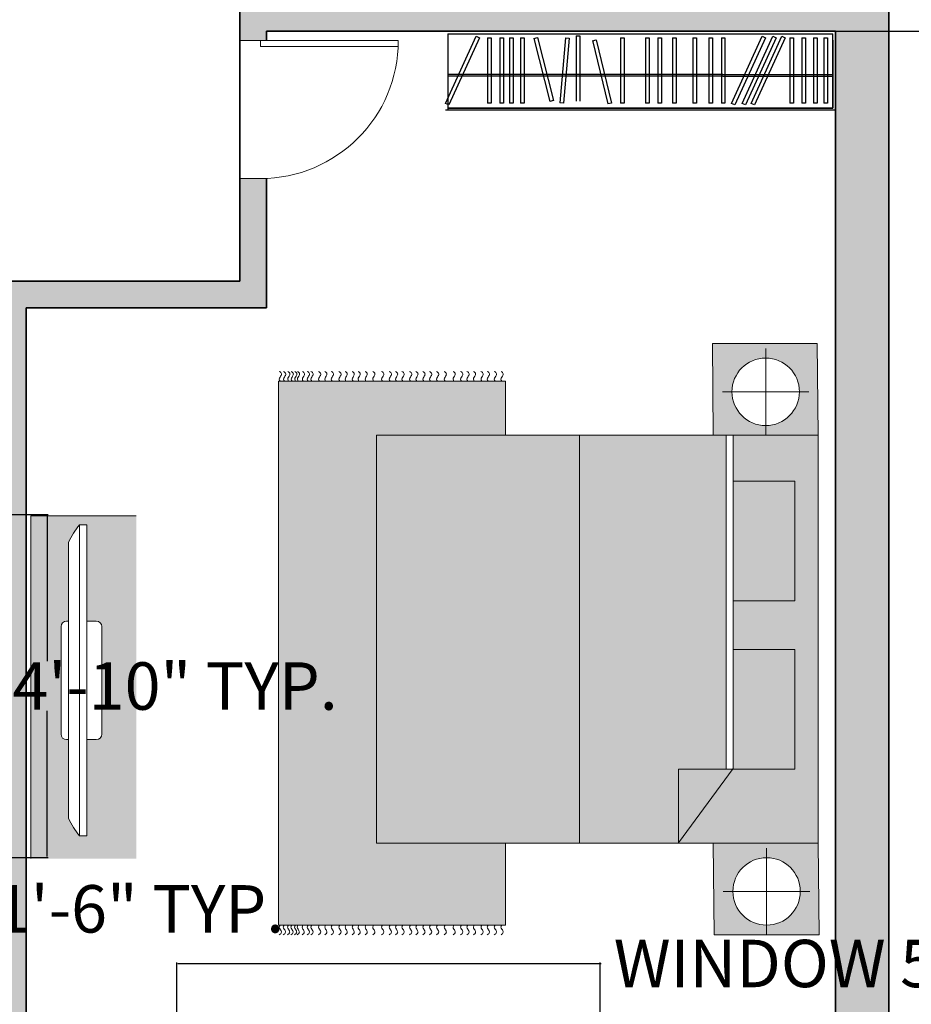
# Model space of a CAD drawing. Units: inches. Extents: x 853 to 1550, y 485 to 1596.
# Tile 7 of 18: x 1267 to 1418, y 867 to 1034. Entities that reach past the tile are written whole.
import ezdxf

# ---------------------------------------------------------------- set-up
doc = ezdxf.new("R2010")
doc.units = ezdxf.units.IN
doc.header["$MEASUREMENT"] = 0
for name, color, linetype, lineweight in [('A-ANNO-DIMS', 2, 'Continuous', 18), ('A-DOOR', 4, 'Continuous', 18), ('A-WALL-PATT', 250, 'Continuous', 13), ('closet', 32, 'Continuous', 25), ('furniture', 250, 'Continuous', 18), ('walls', 250, 'Continuous', 35)]:
    doc.layers.add(name, color=color, linetype=linetype, lineweight=lineweight)
doc.layers.add('A-FURN-PATT', color=254, linetype='Continuous', lineweight=13, true_color=0xfeeab9)
doc.styles.get("Standard").update_dxf_attribs({"font": 'arial.ttf'})
doc.dimstyles.get("Standard").update_dxf_attribs({"dimtxt": 8, "dimasz": 0.18, "dimexe": 0.18, "dimexo": 0.0625, "dimgap": 0.09, "dimtad": 0, "dimtih": 1, "dimtoh": 1, "dimzin": 0, "dimdsep": 46, "dimlunit": 3, "dimtxsty": 'Standard', "dimcen": 0.09, "dimadec": 0, "dimazin": 0, "dimtfac": 1, "dimtofl": 0, "dimtmove": 0, "dimatfit": 3, "dimfxl": 1, "dimtolj": 1, "dimtzin": 0, "dimarcsym": 0})

# ---------------------------------------------------------------- blocks, each defined once
blk = doc.blocks.new('CARPET')
at = {"layer": 'furniture'}
for p, q in [((-51.53, -98.11), (-51.53, -55.12)), ((-51.53, -55.12), (-41.27, -55.12)), ((36, -55.12), (51.55, -55.12)), ((51.55, -55.12), (51.55, -98.11)), ((51.55, -98.11), (-51.53, -98.11))]:
    blk.add_line(p, q, dxfattribs=at)
for points, knots in [([(-53.37, -55.99), (-53.22, -55.8), (-52.9, -55.41), (-52.34, -55.8), (-51.89, -56.08), (-51.65, -55.91), (-51.53, -55.83)], [0, 0, 0, 0, 0.653278, 1.290138, 1.740457, 2.114451, 2.114451, 2.114451, 2.114451]), ([(53.37, -55.99), (53.22, -55.8), (52.9, -55.41), (52.34, -55.8), (51.89, -56.08), (51.65, -55.91), (51.53, -55.83)], [0, 0, 0, 0, 0.653278, 1.290138, 1.740457, 2.114451, 2.114451, 2.114451, 2.114451]), ([(-53.37, -57.26), (-53.22, -57.07), (-52.9, -56.67), (-52.34, -57.07), (-51.89, -57.35), (-51.65, -57.17), (-51.53, -57.1)], [0, 0, 0, 0, 0.653278, 1.290138, 1.740457, 2.114451, 2.114451, 2.114451, 2.114451]), ([(53.37, -57.26), (53.22, -57.07), (52.9, -56.67), (52.34, -57.07), (51.89, -57.35), (51.65, -57.17), (51.53, -57.1)], [0, 0, 0, 0, 0.653278, 1.290138, 1.740457, 2.114451, 2.114451, 2.114451, 2.114451]), ([(-53.37, -58.59), (-53.22, -58.4), (-52.9, -58.01), (-52.34, -58.4), (-51.89, -58.68), (-51.65, -58.5), (-51.53, -58.43)], [0, 0, 0, 0, 0.653278, 1.290138, 1.740457, 2.114451, 2.114451, 2.114451, 2.114451]), ([(-53.37, -59.78), (-53.22, -59.58), (-52.9, -59.19), (-52.34, -59.58), (-51.89, -59.86), (-51.65, -59.69), (-51.53, -59.61)], [0, 0, 0, 0, 0.653278, 1.290138, 1.740457, 2.114451, 2.114451, 2.114451, 2.114451]), ([(53.37, -58.59), (53.22, -58.4), (52.9, -58.01), (52.34, -58.4), (51.89, -58.68), (51.65, -58.5), (51.53, -58.43)], [0, 0, 0, 0, 0.653278, 1.290138, 1.740457, 2.114451, 2.114451, 2.114451, 2.114451]), ([(53.37, -59.78), (53.22, -59.58), (52.9, -59.19), (52.34, -59.58), (51.89, -59.86), (51.65, -59.69), (51.53, -59.61)], [0, 0, 0, 0, 0.653278, 1.290138, 1.740457, 2.114451, 2.114451, 2.114451, 2.114451]), ([(-53.37, -61.22), (-53.22, -61.02), (-52.9, -60.63), (-52.34, -61.02), (-51.89, -61.3), (-51.65, -61.13), (-51.53, -61.05)], [0, 0, 0, 0, 0.653278, 1.290138, 1.740457, 2.114451, 2.114451, 2.114451, 2.114451]), ([(53.37, -61.22), (53.22, -61.02), (52.9, -60.63), (52.34, -61.02), (51.89, -61.3), (51.65, -61.13), (51.53, -61.05)], [0, 0, 0, 0, 0.653278, 1.290138, 1.740457, 2.114451, 2.114451, 2.114451, 2.114451]), ([(-53.37, -62.44), (-53.22, -62.25), (-52.9, -61.86), (-52.34, -62.25), (-51.89, -62.53), (-51.65, -62.36), (-51.53, -62.28)], [0, 0, 0, 0, 0.653278, 1.290138, 1.740457, 2.114451, 2.114451, 2.114451, 2.114451]), ([(-53.37, -63.63), (-53.22, -63.43), (-52.9, -63.04), (-52.34, -63.43), (-51.89, -63.72), (-51.65, -63.54), (-51.53, -63.46)], [0, 0, 0, 0, 0.653278, 1.290138, 1.740457, 2.114451, 2.114451, 2.114451, 2.114451]), ([(53.37, -62.44), (53.22, -62.25), (52.9, -61.86), (52.34, -62.25), (51.89, -62.53), (51.65, -62.36), (51.53, -62.28)], [0, 0, 0, 0, 0.653278, 1.290138, 1.740457, 2.114451, 2.114451, 2.114451, 2.114451]), ([(53.37, -63.63), (53.22, -63.43), (52.9, -63.04), (52.34, -63.43), (51.89, -63.72), (51.65, -63.54), (51.53, -63.46)], [0, 0, 0, 0, 0.653278, 1.290138, 1.740457, 2.114451, 2.114451, 2.114451, 2.114451]), ([(-53.37, -65.07), (-53.22, -64.87), (-52.9, -64.48), (-52.34, -64.87), (-51.89, -65.15), (-51.65, -64.98), (-51.53, -64.9)], [0, 0, 0, 0, 0.653278, 1.290138, 1.740457, 2.114451, 2.114451, 2.114451, 2.114451]), ([(53.37, -65.07), (53.22, -64.87), (52.9, -64.48), (52.34, -64.87), (51.89, -65.15), (51.65, -64.98), (51.53, -64.9)], [0, 0, 0, 0, 0.653278, 1.290138, 1.740457, 2.114451, 2.114451, 2.114451, 2.114451]), ([(-53.37, -66.76), (-53.22, -66.56), (-52.9, -66.17), (-52.34, -66.56), (-51.89, -66.84), (-51.65, -66.67), (-51.53, -66.59)], [0, 0, 0, 0, 0.653278, 1.290138, 1.740457, 2.114451, 2.114451, 2.114451, 2.114451]), ([(53.37, -66.76), (53.22, -66.56), (52.9, -66.17), (52.34, -66.56), (51.89, -66.84), (51.65, -66.67), (51.53, -66.59)], [0, 0, 0, 0, 0.653278, 1.290138, 1.740457, 2.114451, 2.114451, 2.114451, 2.114451]), ([(-53.37, -68.2), (-53.22, -68), (-52.9, -67.61), (-52.34, -68), (-51.89, -68.28), (-51.65, -68.11), (-51.53, -68.03)], [0, 0, 0, 0, 0.653278, 1.290138, 1.740457, 2.114451, 2.114451, 2.114451, 2.114451]), ([(53.37, -68.2), (53.22, -68), (52.9, -67.61), (52.34, -68), (51.89, -68.28), (51.65, -68.11), (51.53, -68.03)], [0, 0, 0, 0, 0.653278, 1.290138, 1.740457, 2.114451, 2.114451, 2.114451, 2.114451]), ([(-53.37, -69.53), (-53.22, -69.33), (-52.9, -68.94), (-52.34, -69.33), (-51.89, -69.61), (-51.65, -69.44), (-51.53, -69.36)], [0, 0, 0, 0, 0.653278, 1.290138, 1.740457, 2.114451, 2.114451, 2.114451, 2.114451]), ([(-53.37, -70.79), (-53.22, -70.6), (-52.9, -70.21), (-52.34, -70.6), (-51.89, -70.88), (-51.65, -70.7), (-51.53, -70.63)], [0, 0, 0, 0, 0.653278, 1.290138, 1.740457, 2.114451, 2.114451, 2.114451, 2.114451]), ([(53.37, -69.53), (53.22, -69.33), (52.9, -68.94), (52.34, -69.33), (51.89, -69.61), (51.65, -69.44), (51.53, -69.36)], [0, 0, 0, 0, 0.653278, 1.290138, 1.740457, 2.114451, 2.114451, 2.114451, 2.114451]), ([(53.37, -70.79), (53.22, -70.6), (52.9, -70.21), (52.34, -70.6), (51.89, -70.88), (51.65, -70.7), (51.53, -70.63)], [0, 0, 0, 0, 0.653278, 1.290138, 1.740457, 2.114451, 2.114451, 2.114451, 2.114451]), ([(-53.37, -72.12), (-53.22, -71.93), (-52.9, -71.54), (-52.34, -71.93), (-51.89, -72.21), (-51.65, -72.04), (-51.53, -71.96)], [0, 0, 0, 0, 0.653278, 1.290138, 1.740457, 2.114451, 2.114451, 2.114451, 2.114451]), ([(53.37, -72.12), (53.22, -71.93), (52.9, -71.54), (52.34, -71.93), (51.89, -72.21), (51.65, -72.04), (51.53, -71.96)], [0, 0, 0, 0, 0.653278, 1.290138, 1.740457, 2.114451, 2.114451, 2.114451, 2.114451]), ([(-53.37, -73.31), (-53.22, -73.11), (-52.9, -72.72), (-52.34, -73.11), (-51.89, -73.4), (-51.65, -73.22), (-51.53, -73.14)], [0, 0, 0, 0, 0.653278, 1.290138, 1.740457, 2.114451, 2.114451, 2.114451, 2.114451]), ([(-53.37, -74.75), (-53.22, -74.55), (-52.9, -74.16), (-52.34, -74.55), (-51.89, -74.83), (-51.65, -74.66), (-51.53, -74.58)], [0, 0, 0, 0, 0.653278, 1.290138, 1.740457, 2.114451, 2.114451, 2.114451, 2.114451]), ([(53.37, -73.31), (53.22, -73.11), (52.9, -72.72), (52.34, -73.11), (51.89, -73.4), (51.65, -73.22), (51.53, -73.14)], [0, 0, 0, 0, 0.653278, 1.290138, 1.740457, 2.114451, 2.114451, 2.114451, 2.114451]), ([(53.37, -74.75), (53.22, -74.55), (52.9, -74.16), (52.34, -74.55), (51.89, -74.83), (51.65, -74.66), (51.53, -74.58)], [0, 0, 0, 0, 0.653278, 1.290138, 1.740457, 2.114451, 2.114451, 2.114451, 2.114451]), ([(-53.37, -75.98), (-53.22, -75.78), (-52.9, -75.39), (-52.34, -75.78), (-51.89, -76.06), (-51.65, -75.89), (-51.53, -75.81)], [0, 0, 0, 0, 0.653278, 1.290138, 1.740457, 2.114451, 2.114451, 2.114451, 2.114451]), ([(53.37, -75.98), (53.22, -75.78), (52.9, -75.39), (52.34, -75.78), (51.89, -76.06), (51.65, -75.89), (51.53, -75.81)], [0, 0, 0, 0, 0.653278, 1.290138, 1.740457, 2.114451, 2.114451, 2.114451, 2.114451]), ([(-53.37, -77.16), (-53.22, -76.96), (-52.9, -76.57), (-52.34, -76.96), (-51.89, -77.25), (-51.65, -77.07), (-51.53, -76.99)], [0, 0, 0, 0, 0.653278, 1.290138, 1.740457, 2.114451, 2.114451, 2.114451, 2.114451]), ([(-53.37, -78.6), (-53.22, -78.4), (-52.9, -78.01), (-52.34, -78.4), (-51.89, -78.68), (-51.65, -78.51), (-51.53, -78.43)], [0, 0, 0, 0, 0.653278, 1.290138, 1.740457, 2.114451, 2.114451, 2.114451, 2.114451]), ([(53.37, -77.16), (53.22, -76.96), (52.9, -76.57), (52.34, -76.96), (51.89, -77.25), (51.65, -77.07), (51.53, -76.99)], [0, 0, 0, 0, 0.653278, 1.290138, 1.740457, 2.114451, 2.114451, 2.114451, 2.114451]), ([(53.37, -78.6), (53.22, -78.4), (52.9, -78.01), (52.34, -78.4), (51.89, -78.68), (51.65, -78.51), (51.53, -78.43)], [0, 0, 0, 0, 0.653278, 1.290138, 1.740457, 2.114451, 2.114451, 2.114451, 2.114451]), ([(-53.37, -80.29), (-53.22, -80.09), (-52.9, -79.7), (-52.34, -80.09), (-51.89, -80.37), (-51.65, -80.2), (-51.53, -80.12)], [0, 0, 0, 0, 0.653278, 1.290138, 1.740457, 2.114451, 2.114451, 2.114451, 2.114451]), ([(53.37, -80.29), (53.22, -80.09), (52.9, -79.7), (52.34, -80.09), (51.89, -80.37), (51.65, -80.2), (51.53, -80.12)], [0, 0, 0, 0, 0.653278, 1.290138, 1.740457, 2.114451, 2.114451, 2.114451, 2.114451]), ([(-53.37, -81.73), (-53.22, -81.53), (-52.9, -81.14), (-52.34, -81.53), (-51.89, -81.81), (-51.65, -81.64), (-51.53, -81.56)], [0, 0, 0, 0, 0.653278, 1.290138, 1.740457, 2.114451, 2.114451, 2.114451, 2.114451]), ([(53.37, -81.73), (53.22, -81.53), (52.9, -81.14), (52.34, -81.53), (51.89, -81.81), (51.65, -81.64), (51.53, -81.56)], [0, 0, 0, 0, 0.653278, 1.290138, 1.740457, 2.114451, 2.114451, 2.114451, 2.114451]), ([(-53.37, -83.06), (-53.22, -82.86), (-52.9, -82.47), (-52.34, -82.86), (-51.89, -83.14), (-51.65, -82.97), (-51.53, -82.89)], [0, 0, 0, 0, 0.653278, 1.290138, 1.740457, 2.114451, 2.114451, 2.114451, 2.114451]), ([(-53.37, -84.18), (-53.22, -83.99), (-52.9, -83.6), (-52.34, -83.99), (-51.89, -84.27), (-51.65, -84.09), (-51.53, -84.02)], [0, 0, 0, 0, 0.653278, 1.290138, 1.740457, 2.114451, 2.114451, 2.114451, 2.114451]), ([(53.37, -83.06), (53.22, -82.86), (52.9, -82.47), (52.34, -82.86), (51.89, -83.14), (51.65, -82.97), (51.53, -82.89)], [0, 0, 0, 0, 0.653278, 1.290138, 1.740457, 2.114451, 2.114451, 2.114451, 2.114451]), ([(53.37, -84.18), (53.22, -83.99), (52.9, -83.6), (52.34, -83.99), (51.89, -84.27), (51.65, -84.09), (51.53, -84.02)], [0, 0, 0, 0, 0.653278, 1.290138, 1.740457, 2.114451, 2.114451, 2.114451, 2.114451]), ([(-53.37, -85.51), (-53.22, -85.32), (-52.9, -84.93), (-52.34, -85.32), (-51.89, -85.6), (-51.65, -85.42), (-51.53, -85.35)], [0, 0, 0, 0, 0.653278, 1.290138, 1.740457, 2.114451, 2.114451, 2.114451, 2.114451]), ([(53.37, -85.51), (53.22, -85.32), (52.9, -84.93), (52.34, -85.32), (51.89, -85.6), (51.65, -85.42), (51.53, -85.35)], [0, 0, 0, 0, 0.653278, 1.290138, 1.740457, 2.114451, 2.114451, 2.114451, 2.114451]), ([(-53.37, -86.7), (-53.22, -86.5), (-52.9, -86.11), (-52.34, -86.5), (-51.89, -86.78), (-51.65, -86.61), (-51.53, -86.53)], [0, 0, 0, 0, 0.653278, 1.290138, 1.740457, 2.114451, 2.114451, 2.114451, 2.114451]), ([(53.37, -86.7), (53.22, -86.5), (52.9, -86.11), (52.34, -86.5), (51.89, -86.78), (51.65, -86.61), (51.53, -86.53)], [0, 0, 0, 0, 0.653278, 1.290138, 1.740457, 2.114451, 2.114451, 2.114451, 2.114451]), ([(-53.37, -88.14), (-53.22, -87.94), (-52.9, -87.55), (-52.34, -87.94), (-51.89, -88.22), (-51.65, -88.05), (-51.53, -87.97)], [0, 0, 0, 0, 0.653278, 1.290138, 1.740457, 2.114451, 2.114451, 2.114451, 2.114451]), ([(-53.37, -89.36), (-53.22, -89.17), (-52.9, -88.78), (-52.34, -89.17), (-51.89, -89.45), (-51.65, -89.28), (-51.53, -89.2)], [0, 0, 0, 0, 0.653278, 1.290138, 1.740457, 2.114451, 2.114451, 2.114451, 2.114451]), ([(53.37, -88.14), (53.22, -87.94), (52.9, -87.55), (52.34, -87.94), (51.89, -88.22), (51.65, -88.05), (51.53, -87.97)], [0, 0, 0, 0, 0.653278, 1.290138, 1.740457, 2.114451, 2.114451, 2.114451, 2.114451]), ([(53.37, -89.36), (53.22, -89.17), (52.9, -88.78), (52.34, -89.17), (51.89, -89.45), (51.65, -89.28), (51.53, -89.2)], [0, 0, 0, 0, 0.653278, 1.290138, 1.740457, 2.114451, 2.114451, 2.114451, 2.114451]), ([(-53.37, -90.55), (-53.22, -90.35), (-52.9, -89.96), (-52.34, -90.35), (-51.89, -90.64), (-51.65, -90.46), (-51.53, -90.38)], [0, 0, 0, 0, 0.653278, 1.290138, 1.740457, 2.114451, 2.114451, 2.114451, 2.114451]), ([(53.37, -90.55), (53.22, -90.35), (52.9, -89.96), (52.34, -90.35), (51.9, -90.63), (51.66, -90.47), (51.55, -90.4)], [0, 0, 0, 0, 0.653278, 1.290138, 1.740457, 2.0926, 2.0926, 2.0926, 2.0926]), ([(-53.37, -91.99), (-53.22, -91.79), (-52.9, -91.4), (-52.34, -91.79), (-51.89, -92.07), (-51.65, -91.9), (-51.53, -91.82)], [0, 0, 0, 0, 0.653278, 1.290138, 1.740457, 2.114451, 2.114451, 2.114451, 2.114451]), ([(-53.37, -92.69), (-53.22, -92.48), (-52.9, -92.08), (-52.35, -92.49), (-51.89, -92.77), (-51.65, -92.6), (-51.53, -92.52)], [0, 0, 0, 0, 0.663904, 1.307406, 1.757725, 2.131719, 2.131719, 2.131719, 2.131719]), ([(-53.37, -93.61), (-53.22, -93.42), (-52.9, -93.03), (-52.34, -93.42), (-51.89, -93.7), (-51.65, -93.52), (-51.53, -93.45)], [0, 0, 0, 0, 0.653278, 1.290138, 1.740457, 2.114451, 2.114451, 2.114451, 2.114451]), ([(53.37, -91.99), (53.22, -91.79), (52.9, -91.4), (52.34, -91.79), (51.9, -92.07), (51.66, -91.91), (51.55, -91.83)], [0, 0, 0, 0, 0.653278, 1.290138, 1.740457, 2.0926, 2.0926, 2.0926, 2.0926]), ([(53.37, -92.69), (53.22, -92.49), (52.9, -92.09), (52.34, -92.49), (51.9, -92.77), (51.66, -92.61), (51.55, -92.53)], [0, 0, 0, 0, 0.656792, 1.295826, 1.746145, 2.098292, 2.098292, 2.098292, 2.098292]), ([(53.37, -93.66), (53.22, -93.46), (52.9, -93.07), (52.34, -93.46), (51.9, -93.74), (51.66, -93.58), (51.55, -93.5)], [0, 0, 0, 0, 0.653278, 1.290138, 1.740457, 2.0926, 2.0926, 2.0926, 2.0926]), ([(-53.37, -94.55), (-53.22, -94.35), (-52.9, -93.96), (-52.34, -94.35), (-51.89, -94.63), (-51.65, -94.46), (-51.53, -94.38)], [0, 0, 0, 0, 0.653278, 1.290138, 1.740457, 2.114451, 2.114451, 2.114451, 2.114451]), ([(-53.37, -95.05), (-53.22, -94.85), (-52.9, -94.46), (-52.34, -94.85), (-51.89, -95.14), (-51.65, -94.96), (-51.53, -94.88)], [0, 0, 0, 0, 0.653278, 1.290138, 1.740457, 2.114451, 2.114451, 2.114451, 2.114451]), ([(53.37, -94.59), (53.22, -94.4), (52.9, -94.01), (52.34, -94.4), (51.9, -94.68), (51.66, -94.51), (51.55, -94.44)], [0, 0, 0, 0, 0.653278, 1.290138, 1.740457, 2.0926, 2.0926, 2.0926, 2.0926]), ([(53.37, -95.1), (53.22, -94.9), (52.9, -94.51), (52.34, -94.9), (51.9, -95.18), (51.66, -95.02), (51.55, -94.94)], [0, 0, 0, 0, 0.653278, 1.290138, 1.740457, 2.0926, 2.0926, 2.0926, 2.0926]), ([(-53.37, -95.73), (-53.22, -95.54), (-52.9, -95.15), (-52.34, -95.54), (-51.89, -95.82), (-51.65, -95.65), (-51.53, -95.57)], [0, 0, 0, 0, 0.653278, 1.290138, 1.740457, 2.114451, 2.114451, 2.114451, 2.114451]), ([(-53.37, -96.38), (-53.22, -96.18), (-52.9, -95.79), (-52.34, -96.18), (-51.89, -96.47), (-51.65, -96.29), (-51.53, -96.21)], [0, 0, 0, 0, 0.653278, 1.290138, 1.740457, 2.114451, 2.114451, 2.114451, 2.114451]), ([(-53.37, -97.17), (-53.22, -96.98), (-52.9, -96.59), (-52.34, -96.98), (-51.89, -97.26), (-51.65, -97.08), (-51.53, -97.01)], [0, 0, 0, 0, 0.653278, 1.290138, 1.740457, 2.114451, 2.114451, 2.114451, 2.114451]), ([(53.37, -95.78), (53.22, -95.58), (52.9, -95.19), (52.34, -95.58), (51.89, -95.86), (51.65, -95.69), (51.53, -95.61)], [0, 0, 0, 0, 0.653278, 1.290138, 1.740457, 2.114451, 2.114451, 2.114451, 2.114451]), ([(53.37, -96.43), (53.22, -96.23), (52.9, -95.84), (52.34, -96.23), (51.89, -96.51), (51.65, -96.34), (51.53, -96.26)], [0, 0, 0, 0, 0.653278, 1.290138, 1.740457, 2.114451, 2.114451, 2.114451, 2.114451]), ([(53.37, -97.22), (53.22, -97.02), (52.9, -96.63), (52.34, -97.02), (51.89, -97.3), (51.65, -97.13), (51.53, -97.05)], [0, 0, 0, 0, 0.653278, 1.290138, 1.740457, 2.114451, 2.114451, 2.114451, 2.114451]), ([(-53.37, -97.99), (-53.22, -97.79), (-52.9, -97.4), (-52.34, -97.79), (-51.89, -98.08), (-51.65, -97.9), (-51.53, -97.82)], [0, 0, 0, 0, 0.653278, 1.290138, 1.740457, 2.114451, 2.114451, 2.114451, 2.114451]), ([(53.37, -97.99), (53.22, -97.79), (52.9, -97.4), (52.34, -97.79), (51.89, -98.08), (51.65, -97.9), (51.53, -97.82)], [0, 0, 0, 0, 0.653278, 1.290138, 1.740457, 2.114451, 2.114451, 2.114451, 2.114451])]:
    blk.add_open_spline(points, degree=3, knots=knots, dxfattribs=at)
blk = doc.blocks.new('A$C58D270C6')
at = {"layer": 'furniture'}
for p, q in [((9.09, 124.13), (9.09, 108.87)), ((1.46, 116.5), (16.73, 116.5)), ((14.97, 94.84), (24.62, 107.92)), ((24.62, 94.93), (24.62, 107.92)), ((42.08, 108), (42.08, 36)), ((14.97, 94.93), (24.62, 94.93)), ((14.97, 94.84), (14.97, 36)), ((16.22, 94.93), (16.22, 36)), ((9.25, 36), (9.25, 20.74)), ((1.62, 28.37), (16.88, 28.37))]:
    blk.add_line(p, q, dxfattribs=at)
for points in [[(18.5, 108), (18.34, 124.13), (-0.16, 124.13), (0, 108)], [(0, 108), (77.91, 108), (77.91, 36), (0, 36)], [(4.09, 94.93), (14.97, 94.93), (14.97, 73.83), (4.09, 73.83)], [(4.09, 65.23), (14.97, 65.23), (14.97, 44.13), (4.09, 44.13)], [(18.65, 19.87), (18.5, 36), (0, 36), (0.16, 19.87)]]:
    blk.add_lwpolyline(points, close=True, dxfattribs=at)
for centre in [(9.09, 116.5), (9.25, 28.37)]:
    blk.add_circle(centre, 5.95, dxfattribs=at)
at = {"layer": 'furniture', "xscale": 0.9312884925094044, "yscale": 0.9312884925094044, "zscale": 0.9312884925094044, "rotation": 90}
blk.add_blockref('CARPET', (3.79, 74.47), dxfattribs=at)
blk = doc.blocks.new('*U10')
for p, q in [((0, 0), (0, -6)), ((40, 0), (40, -6))]:
    blk.add_line(p, q)
blk.add_lwpolyline([(0, 0), (0, 40), (1.75, 40), (1.75, 0)], close=True)
blk.add_arc((0, 0), 40, 0, 90)
blk = doc.blocks.new('closet')
at = {"layer": 'closet'}
for p, q in [((-0.71, -5.58), (5.59, 8.19)), ((5.59, 8.19), (6.27, 7.88)), ((26.09, 8.25), (26.09, -5.1)), ((26.84, 8.25), (26.84, -5.1)), ((57.99, -5.58), (64.3, 8.19)), ((60.19, -5.58), (66.49, 8.19)), ((62, -5.58), (68.3, 8.19)), ((-0.23, 7.39), (-0.23, -6.57)), ((6.27, 7.88), (-0.04, -5.89)), ((7.92, 7.84), (8.68, 7.84)), ((7.92, 7.84), (7.92, -5.51)), ((8.68, 7.84), (8.68, -5.51)), ((10.44, 7.84), (11.2, 7.84)), ((10.44, 7.84), (10.44, -5.51)), ((11.2, 7.84), (11.2, -5.51)), ((12.45, 7.84), (13.21, 7.84)), ((12.45, 7.84), (12.45, -5.51)), ((13.21, 7.84), (13.21, -5.51)), ((14.71, 7.84), (15.47, 7.84)), ((14.71, 7.84), (14.71, -5.51)), ((15.47, 7.84), (15.47, -5.51)), ((17.44, 7.75), (18.17, 7.93)), ((17.44, 7.75), (20.73, -5.2)), ((18.17, 7.93), (21.46, -5.01)), ((23.92, 7.84), (22.75, -5.46)), ((24.67, 7.78), (23.51, -5.53)), ((23.92, 7.84), (24.67, 7.78)), ((29.49, 7.29), (32.64, -5.69)), ((30.22, 7.46), (33.37, -5.51)), ((35.23, 7.84), (35.23, -5.51)), ((35.99, 7.84), (35.99, -5.51)), ((40.33, 7.84), (40.33, -5.51)), ((41.08, 7.84), (41.08, -5.51)), ((42.85, 7.84), (42.85, -5.51)), ((43.61, 7.84), (43.61, -5.51)), ((45.9, 7.84), (45.9, -5.51)), ((46.65, 7.84), (46.65, -5.51)), ((50.07, 7.84), (50.07, -5.51)), ((50.82, 7.84), (50.82, -5.51)), ((53.32, 7.84), (53.32, -5.51)), ((54.08, 7.84), (54.08, -5.51)), ((55.9, 7.84), (55.9, -5.51)), ((56.65, 7.84), (56.65, -5.51)), ((64.97, 7.88), (58.67, -5.89)), ((67.17, 7.88), (60.87, -5.89)), ((68.98, 7.88), (62.67, -5.89)), ((69.96, 7.84), (69.96, -5.51)), ((70.72, 7.84), (70.72, -5.51)), ((72.43, 7.84), (72.43, -5.51)), ((73.19, 7.84), (73.19, -5.51)), ((74.82, 7.84), (74.82, -5.51)), ((75.57, 7.84), (75.57, -5.51)), ((76.94, 7.84), (76.94, -5.51)), ((77.69, 7.84), (77.69, -5.51)), ((56.23, 0.33), (0, 0.33)), ((56.2, 0), (0, 0)), ((56.2, 0), (78.76, 0)), ((56.23, 0.33), (78.76, 0.33)), ((-0.04, -5.89), (-0.71, -5.58)), ((21.46, -5.01), (20.73, -5.2)), ((23.51, -5.53), (22.75, -5.46)), ((33.37, -5.51), (32.64, -5.69)), ((35.99, -5.51), (35.23, -5.51)), ((41.08, -5.51), (40.33, -5.51)), ((43.61, -5.51), (42.85, -5.51)), ((46.65, -5.51), (45.9, -5.51)), ((50.82, -5.51), (50.07, -5.51)), ((54.08, -5.51), (53.32, -5.51)), ((56.65, -5.51), (55.9, -5.51)), ((58.67, -5.89), (57.99, -5.58)), ((60.87, -5.89), (60.19, -5.58)), ((62.67, -5.89), (62, -5.58)), ((70.72, -5.51), (69.96, -5.51)), ((73.19, -5.51), (72.43, -5.51)), ((75.57, -5.51), (74.82, -5.51)), ((77.69, -5.51), (76.94, -5.51))]:
    blk.add_line(p, q, dxfattribs=at)
blk = doc.blocks.new('rotated closet')
at = {"layer": 'closet'}
for p, q in [((26.32, 0.86), (27.07, 0.86)), ((29.72, -0.11), (30.45, 0.07)), ((35.46, 0.45), (36.22, 0.45)), ((40.56, 0.45), (41.31, 0.45)), ((43.08, 0.45), (43.84, 0.45)), ((46.13, 0.45), (46.88, 0.45)), ((50.3, 0.45), (51.05, 0.45)), ((53.56, 0.45), (54.31, 0.45)), ((56.13, 0.45), (56.88, 0.45)), ((64.53, 0.8), (65.2, 0.49)), ((66.72, 0.8), (67.4, 0.49)), ((68.53, 0.8), (69.21, 0.49)), ((70.19, 0.45), (70.95, 0.45)), ((72.66, 0.45), (73.42, 0.45)), ((75.05, 0.45), (75.81, 0.45)), ((77.17, 0.45), (77.92, 0.45)), ((78.99, 0), (78.99, -13.96)), ((0, -13.96), (78.99, -13.96)), ((8.91, -12.91), (8.15, -12.91)), ((11.43, -12.91), (10.67, -12.91)), ((13.44, -12.91), (12.68, -12.91)), ((15.7, -12.91), (14.94, -12.91)), ((-0.46, -14.27), (79.54, -14.27))]:
    blk.add_line(p, q, dxfattribs=at)
blk.add_blockref('closet', (0.23, -7.39), dxfattribs=at)
blk = doc.blocks.new('WARDROBE-FRAMED')
for p, q in [((0.4, 12.8), (65.33, 12.8)), ((0.4, 12.8), (0.4, 0.26)), ((65.33, 0.26), (65.33, 12.8)), ((0.02, 0), (65.79, 0)), ((65.33, 0.26), (0.4, 0.26)), ((0.4, 0.26), (0.4, 0))]:
    blk.add_line(p, q)
at = {"xscale": 0.8221057635095903, "yscale": 0.8221057635095903, "zscale": 0.8221057635095903, "rotation": 359.9999999992008}
blk.add_blockref('rotated closet', (0.4, 11.74), dxfattribs=at)
blk = doc.blocks.new('PLASMA-LARGE')
at = {"layer": 'furniture'}
for p, q in [((-7.26, 0), (7.26, 0)), ((-18.61, -1), (18.61, -1)), ((-8, -1), (-8, -0.74)), ((8, -1), (8, -0.74)), ((-21, -2.5), (21, -2.5)), ((-21, -2.5), (-21, -3.5)), ((21, -2.5), (21, -3.5)), ((-21, -3.5), (21, -3.5)), ((-8, -3.5), (-8, -4.76)), ((8, -3.5), (8, -4.76)), ((-7.26, -5.5), (7.26, -5.5))]:
    blk.add_line(p, q, dxfattribs=at)
for centre, radius, start, end in [((-7.26, -0.74), 0.744, 90, 180), ((7.26, -0.74), 0.744, 0, 90), ((-13.97, -11.05), 11.07, 114.7602, 129.4175), ((13.97, -11.05), 11.07, 50.5825, 65.2398), ((-7.26, -4.76), 0.744, 180, 270), ((7.26, -4.76), 0.744, 270, 0)]:
    blk.add_arc(centre, radius, start, end, dxfattribs=at)
blk = doc.blocks.new('TV-CONSOLE-WALL')
for p, q in [((17.81, 57.83), (0, 57.83)), ((0, 57.83), (0, 0))]:
    blk.add_line(p, q)
at = {"xscale": -1.249763490704796, "yscale": 1.249763490704796, "zscale": 1.249763490704796, "rotation": 90}
blk.add_blockref('PLASMA-LARGE', (5.11, 30.08), dxfattribs=at)
blk = doc.blocks.new('*D41')
at = {"layer": 'A-ANNO-DIMS', "color": 0, "lineweight": -2, "transparency": 16777216}
for p, q in [((1293.81, 863.69), (1293.81, 874.52)), ((1293.99, 874.34), (1365.06, 874.34)), ((1365.24, 863.69), (1365.24, 874.52)), ((1365.24, 874.34), (1365.42, 874.34))]:
    blk.add_line(p, q, dxfattribs=at)
at = {"layer": 'A-ANNO-DIMS', "color": 0, "transparency": 16777216}
for points in [[(1293.99, 874.37), (1293.99, 874.31), (1293.81, 874.34)], [(1365.06, 874.37), (1365.06, 874.31), (1365.24, 874.34)]]:
    blk.add_solid(points, dxfattribs=at)
at = {"layer": 'Defpoints', "color": 0, "transparency": 16777216}
for p in [(1365.24, 874.34), (1293.81, 863.63), (1365.24, 863.63)]:
    blk.add_point(p, dxfattribs=at)
at = {"layer": 'A-ANNO-DIMS', "color": 0, "transparency": 16777216, "insert": (1428.56, 874.34), "char_height": 8, "attachment_point": 5}
blk.add_mtext('\\A1;WINDOW 5\'-11 1/2" TYP.', dxfattribs=at)
blk = doc.blocks.new('*D42')
at = {"layer": 'A-ANNO-DIMS', "color": 0, "lineweight": -2, "transparency": 16777216}
for p, q in [((1293.75, 863.63), (1282.92, 863.63)), ((1283.1, 863.45), (1283.1, 863.3)), ((1293.75, 854.63), (1282.92, 854.63)), ((1283.1, 854.81), (1283.1, 854.95))]:
    blk.add_line(p, q, dxfattribs=at)
at = {"layer": 'A-ANNO-DIMS', "color": 0, "transparency": 16777216}
for points in [[(1283.07, 863.45), (1283.13, 863.45), (1283.1, 863.63)], [(1283.07, 854.81), (1283.13, 854.81), (1283.1, 854.63)]]:
    blk.add_solid(points, dxfattribs=at)
at = {"layer": 'Defpoints', "color": 0, "transparency": 16777216}
for p in [(1283.1, 863.63), (1293.81, 863.63), (1293.81, 854.63)]:
    blk.add_point(p, dxfattribs=at)
at = {"layer": 'A-ANNO-DIMS', "color": 0, "transparency": 16777216, "insert": (1283.1, 859.13), "char_height": 8, "attachment_point": 5}
blk.add_mtext('\\A1;0\'-9" TYP.', dxfattribs=at)
blk = doc.blocks.new('*D45')
at = {"layer": 'A-ANNO-DIMS', "color": 0, "lineweight": -2, "transparency": 16777216}
for p, q in [((1263.33, 950.07), (1272.12, 950.07)), ((1271.94, 949.89), (1271.94, 925.33)), ((1271.94, 892.42), (1271.94, 916.98)), ((1263.33, 892.24), (1272.12, 892.24))]:
    blk.add_line(p, q, dxfattribs=at)
at = {"layer": 'A-ANNO-DIMS', "color": 0, "transparency": 16777216}
for points in [[(1271.91, 949.89), (1271.97, 949.89), (1271.94, 950.07)], [(1271.91, 892.42), (1271.97, 892.42), (1271.94, 892.24)]]:
    blk.add_solid(points, dxfattribs=at)
at = {"layer": 'Defpoints', "color": 0, "transparency": 16777216}
for p in [(1263.27, 950.07), (1271.94, 950.07), (1263.27, 892.24)]:
    blk.add_point(p, dxfattribs=at)
at = {"layer": 'A-ANNO-DIMS', "color": 0, "transparency": 16777216, "insert": (1271.94, 921.15), "char_height": 8, "attachment_point": 5}
blk.add_mtext('\\A1;TV UNIT 4\'-10" TYP.', dxfattribs=at)
blk = doc.blocks.new('*D46')
at = {"layer": 'A-ANNO-DIMS', "color": 0, "lineweight": -2, "transparency": 16777216}
for p, q in [((1245.45, 892.17), (1245.45, 883.38)), ((1263.27, 892.17), (1263.27, 883.38)), ((1245.63, 883.56), (1263.09, 883.56)), ((1263.27, 883.56), (1263.45, 883.56))]:
    blk.add_line(p, q, dxfattribs=at)
at = {"layer": 'A-ANNO-DIMS', "color": 0, "transparency": 16777216}
for points in [[(1245.63, 883.59), (1245.63, 883.53), (1245.45, 883.56)], [(1263.09, 883.59), (1263.09, 883.53), (1263.27, 883.56)]]:
    blk.add_solid(points, dxfattribs=at)
at = {"layer": 'Defpoints', "color": 0, "transparency": 16777216}
for p in [(1245.45, 892.24), (1263.27, 892.24), (1263.27, 883.56)]:
    blk.add_point(p, dxfattribs=at)
at = {"layer": 'A-ANNO-DIMS', "color": 0, "transparency": 16777216, "insert": (1287.54, 883.56), "char_height": 8, "attachment_point": 5}
blk.add_mtext('\\A1;1\'-6" TYP.', dxfattribs=at)
blk = doc.blocks.new('*D75')
at = {"layer": 'A-ANNO-DIMS', "color": 0, "lineweight": -2, "transparency": 16777216}
for p, q in [((1405, 1031.63), (1526.24, 1031.63)), ((1526.06, 1031.45), (1526.06, 951.8)), ((1526.06, 863.81), (1526.06, 943.45)), ((1405, 863.63), (1526.24, 863.63))]:
    blk.add_line(p, q, dxfattribs=at)
at = {"layer": 'A-ANNO-DIMS', "color": 0, "transparency": 16777216}
for points in [[(1526.03, 1031.45), (1526.09, 1031.45), (1526.06, 1031.63)], [(1526.03, 863.81), (1526.09, 863.81), (1526.06, 863.63)]]:
    blk.add_solid(points, dxfattribs=at)
at = {"layer": 'Defpoints', "color": 0, "transparency": 16777216}
for p in [(1404.94, 1031.63), (1526.06, 1031.63), (1404.94, 863.63)]:
    blk.add_point(p, dxfattribs=at)
at = {"layer": 'A-ANNO-DIMS', "color": 0, "transparency": 16777216, "insert": (1526.06, 947.63), "char_height": 8, "attachment_point": 5}
blk.add_mtext('\\A1;14\'-0"', dxfattribs=at)

msp = doc.modelspace()

# ---------------------------------------------------------------- hatches: boundary and pattern name
at = {"layer": 'A-FURN-PATT'}
h = msp.add_hatch(color=256, dxfattribs=at)
h.dxf.hatch_style = 1
h.paths.add_polyline_path([(1387.693, 963.493), (1402.014, 963.493), (1402.014, 894.632), (1378.471, 894.632), (1378.471, 894.706), (1387.631, 907.13), (1398.098, 907.13), (1398.098, 927.307), (1387.693, 927.307), (1387.693, 935.54), (1398.098, 935.54), (1398.098, 955.717), (1387.693, 955.717)])
h.paths.add_polyline_path([(1378.471, 907.13), (1387.631, 907.13), (1378.471, 894.706)], flags=17)
h.paths.add_polyline_path([(1387.621, 886.503, 0.4142136), (1393.317, 880.807), (1393.317, 879.204), (1384.47, 879.204), (1384.322, 894.632), (1402.014, 894.632), (1402.163, 879.204), (1393.317, 879.204), (1393.317, 880.807, 0.4142136), (1399.012, 886.503, 1)])
h.paths.add_polyline_path([(1384.173, 978.92), (1401.865, 978.92), (1402.014, 963.493), (1393.168, 963.493), (1393.168, 965.096, 0.4142136), (1398.863, 970.791, 1), (1387.473, 970.791, 0.4142136), (1393.168, 965.096), (1393.168, 963.493), (1384.322, 963.493)])
h = msp.add_hatch(color=256, dxfattribs=at)
h.dxf.hatch_style = 1
h.paths.add_polyline_path([(1311.005, 972.598), (1349.291, 972.598), (1349.291, 963.493), (1327.506, 963.493), (1327.506, 894.632), (1349.291, 894.632), (1349.291, 880.78), (1311.005, 880.78)])
h.paths.add_polyline_path([(1363.837, 911.44), (1321.629, 911.44), (1321.629, 922.311), (1363.837, 922.311)], flags=9)
h.paths.add_polyline_path([(1363.89, 923.509), (1301.93, 923.509), (1301.93, 934.698), (1363.89, 934.698)], flags=9)
h = msp.add_hatch(color=256, dxfattribs=at)
h.dxf.hatch_style = 1
h.paths.add_polyline_path([(1311.005, 972.598), (1349.291, 972.598), (1349.291, 963.493), (1327.506, 963.493), (1327.506, 894.632), (1349.291, 894.632), (1349.291, 880.78), (1311.005, 880.78)])
h = msp.add_hatch(color=256, dxfattribs=at)
h.dxf.hatch_style = 1
h.paths.add_polyline_path([(1327.506, 963.493), (1361.771, 963.493), (1361.771, 894.632), (1327.506, 894.632)])
h.paths.add_polyline_path([(1361.771, 963.493), (1386.504, 963.493), (1386.504, 907.13), (1378.471, 907.13), (1378.471, 894.632), (1361.771, 894.632)])
h = msp.add_hatch(color=256, dxfattribs=at)
h.dxf.hatch_style = 1
h.paths.add_polyline_path([(1387.693, 927.307), (1398.098, 927.307), (1398.098, 907.13), (1387.693, 907.13)])
h.paths.add_polyline_path([(1387.693, 955.717), (1398.098, 955.717), (1398.098, 935.54), (1387.693, 935.54)])
h = msp.add_hatch(color=256, dxfattribs=at)
h.dxf.hatch_style = 1
h.paths.add_polyline_path([(1287.006, 949.861), (1287.006, 892.028), (1269.194, 892.028), (1269.194, 949.861)])
h.paths.add_polyline_path([(1281.173, 931.18, 0.4142136), (1280.243, 932.11), (1278.674, 932.11), (1278.674, 948.357), (1277.424, 948.357, 0.0640419), (1275.549, 945.368), (1275.549, 932.11), (1275.23, 932.11, 0.4142136), (1274.299, 931.18), (1274.299, 913.044, 0.4142136), (1275.23, 912.114), (1275.549, 912.114), (1275.549, 898.857, 0.0640419), (1277.424, 895.867), (1278.674, 895.867), (1278.674, 912.114), (1280.243, 912.114, 0.4142136), (1281.173, 913.044)], flags=16)
at = {"layer": 'A-WALL-PATT'}
h = msp.add_hatch(color=256, dxfattribs=at)
h.dxf.hatch_style = 1
h.paths.add_polyline_path([(1139.437, 988.732), (1134.937, 988.732), (1134.937, 830.473), (1139.437, 830.473)])
h.paths.add_polyline_path([(1413.937, 1052.227), (1404.937, 1052.227), (1404.937, 1036.129), (1308.937, 1036.129), (1308.937, 1045.033), (1304.437, 1045.033), (1304.437, 1030.033), (1308.937, 1030.033), (1308.937, 1031.629), (1404.937, 1031.629), (1404.937, 863.629), (1365.241, 863.629), (1365.241, 854.629), (1413.937, 854.629)])
h.paths.add_polyline_path([(1413.937, 1133.918), (1404.937, 1133.918), (1404.937, 1100.629), (1304.437, 1100.629), (1304.437, 1078.26), (1308.937, 1078.26), (1308.937, 1096.129), (1404.937, 1096.129), (1404.937, 1084.233), (1407.946, 1084.233), (1413.937, 1084.233)])
h.paths.add_polyline_path([(1268.437, 1417.129), (1288.974, 1417.129), (1288.974, 1426.129), (1244.597, 1426.129), (1244.597, 1417.129), (1263.937, 1417.129), (1263.937, 1321.129), (1260.34, 1321.129), (1260.34, 1316.629), (1263.937, 1316.629), (1263.937, 1283.505), (1268.437, 1283.505)])
h.paths.add_polyline_path([(1413.937, 1426.129), (1360.402, 1426.129), (1360.402, 1417.129), (1404.937, 1417.129), (1404.937, 1249.129), (1268.437, 1249.129), (1268.437, 1254.041), (1268.357, 1254.041), (1263.937, 1254.041), (1263.937, 1244.629), (1404.937, 1244.629), (1404.937, 1228.163), (1413.937, 1228.163)])
h.paths.add_polyline_path([(1215.842, 1426.129), (1184.201, 1426.129), (1184.201, 1417.129), (1199.437, 1417.129), (1199.437, 1321.129), (1172.101, 1321.129), (1172.101, 1316.629), (1229.433, 1316.629), (1229.433, 1321.129), (1203.937, 1321.129), (1203.937, 1417.129), (1215.842, 1417.129)])
h.paths.add_polyline_path([(1139.437, 1417.129), (1155.446, 1417.129), (1155.446, 1426.129), (1091.831, 1426.129), (1091.831, 1417.129), (1134.937, 1417.129), (1134.937, 1289.22), (1139.437, 1289.22), (1139.437, 1316.629), (1143.553, 1316.629), (1143.553, 1321.129), (1139.437, 1321.129)])
h.paths.add_polyline_path([(1139.437, 1255.161), (1134.937, 1255.161), (1134.937, 1249.129), (990.937, 1249.129), (990.937, 1417.129), (1020.402, 1417.129), (1020.402, 1426.129), (981.937, 1426.129), (981.937, 1205.535), (984.477, 1205.535), (990.937, 1205.535), (990.937, 1244.629), (1134.937, 1244.629), (1134.937, 1237.775), (1139.437, 1237.775)])
h = msp.add_hatch(color=256, dxfattribs=at)
h.dxf.hatch_style = 1
h.paths.add_polyline_path([(990.937, 1111.29), (981.937, 1111.29), (981.937, 1044.136), (984.946, 1044.136), (990.937, 1044.136), (990.937, 1072.129), (1045.609, 1072.129, -0.0272078), (1045.453, 1074.983), (1045.453, 1076.629), (990.937, 1076.629)], flags=17)
h.paths.add_polyline_path([(1091.437, 1072.129), (1139.437, 1072.129), (1139.437, 1206.521), (1134.937, 1206.521), (1134.937, 1076.629), (1071.734, 1076.629), (1071.734, 1074.983), (1071.734, 1072.129), (1086.937, 1072.129), (1086.937, 1012.129), (990.937, 1012.129), (981.937, 1012.129), (981.937, 944.409), (990.937, 944.409), (990.937, 1007.629), (1091.437, 1007.629)])
h.paths.add_polyline_path([(990.937, 872.981), (981.937, 872.981), (981.937, 788.629), (990.937, 788.629)])
h.paths.add_polyline_path([(1014.605, 800.886), (990.937, 800.886), (990.937, 796.386), (1014.605, 796.386)])
h.paths.add_polyline_path([(1134.937, 793.129), (1090.727, 793.129), (1090.727, 788.629), (1134.937, 788.629)])
h.paths.add_polyline_path([(1139.437, 800.892), (1134.937, 800.892), (1134.937, 788.629), (1113.94, 788.629), (1113.94, 767.629), (1139.437, 767.629), (1191.938, 767.629), (1191.938, 772.657), (1191.938, 776.629), (1139.437, 776.629)])
h.paths.add_polyline_path([(1131.331, 781.621), (1131.331, 775.236), (1118.809, 775.236), (1118.809, 781.621)], flags=16)
h.paths.add_polyline_path([(1131.331, 781.621), (1118.809, 781.621), (1118.809, 775.236), (1131.331, 775.236)], flags=0)
h.paths.add_polyline_path([(1118.963, 707.356), (1110.94, 707.356), (1110.94, 699.868), (1118.963, 699.868)])
h.paths.add_polyline_path([(1284.919, 707.356), (1276.896, 707.356), (1276.896, 699.868), (1284.919, 699.868)])
h.paths.add_polyline_path([(1293.812, 863.629), (1268.437, 863.629), (1268.437, 984.936), (1308.937, 984.936), (1308.937, 996.627), (1304.437, 996.627), (1304.437, 989.436), (1263.937, 989.436), (1263.937, 863.629), (1215.364, 863.629), (1215.364, 854.629), (1252.179, 854.629), (1252.179, 776.629), (1225.216, 776.629, -0.0297134), (1225.453, 772.657), (1225.453, 767.629), (1261.179, 767.629), (1261.179, 854.629), (1293.812, 854.629)])
h.paths.add_polyline_path([(1176.151, 863.629), (1139.437, 863.629), (1139.437, 854.629), (1176.151, 854.629)])
h.paths.add_polyline_path([(1134.937, 863.629), (1109.834, 863.629), (1109.834, 859.129), (1134.937, 859.129)])
h.paths.add_polyline_path([(1148.879, 950.672), (1144.374, 950.672), (1144.374, 874.094), (1148.879, 874.094)])
h.paths.add_polyline_path([(1079.778, 863.629), (990.937, 863.629), (990.937, 859.129), (1079.778, 859.129)])
h = msp.add_hatch(color=256, dxfattribs=at)
h.dxf.hatch_style = 1
h.paths.add_polyline_path([(1308.937, 1006.784, -0.0108475), (1307.928, 1006.762), (1304.437, 1006.762), (1304.437, 996.642), (1308.937, 996.642)])

# ---------------------------------------------------------------- linework, layer by layer
at = {"layer": 'walls'}
for p, q in [((1413.937, 1426.129), (1413.937, 854.629)), ((1304.437, 1100.629), (1304.437, 989.436)), ((1308.937, 1031.629), (1404.937, 1031.629)), ((1308.937, 1031.629), (1308.937, 1030.033)), ((1404.937, 1031.629), (1404.937, 863.629)), ((1308.937, 1006.784), (1308.937, 984.936)), ((1263.937, 989.436), (1304.437, 989.436)), ((1268.437, 863.629), (1268.437, 984.936)), ((1268.437, 984.936), (1308.937, 984.936))]:
    msp.add_line(p, q, dxfattribs=at)

# ---------------------------------------------------------------- block references
at = {"layer": 'A-DOOR', "xscale": 0.581772061012954, "yscale": 0.581772061012954, "zscale": 0.581772061012954, "rotation": 270}
msp.add_blockref('*U10', (1307.928, 1030.033), dxfattribs=at)
at = {"layer": 'closet'}
msp.add_blockref('WARDROBE-FRAMED', (1339.142, 1018.371), dxfattribs=at)
at = {"layer": 'furniture', "xscale": 0.9563987329230524, "yscale": 0.9563987329230524, "zscale": 0.9563987329230524, "rotation": 180}
msp.add_blockref('A$C58D270C6', (1402.014, 997.923), dxfattribs=at)
at = {"layer": 'furniture'}
msp.add_blockref('TV-CONSOLE-WALL', (1269.194, 892.028), dxfattribs=at)

# ---------------------------------------------------------------- dimensions: what is measured, and where the dimension line sits
at = {"layer": 'A-ANNO-DIMS'}
dim = msp.add_linear_dim(base=(1526.064, 1031.629), p1=(1404.937, 863.629), p2=(1404.937, 1031.629), angle=90, dimstyle='Standard', override={"dimdec": 1, "dimlfac": 1, "dimrnd": 0, "dimzin": 1, "dimdsep": 46, "dimlunit": 4, "dimfrac": 2}, dxfattribs=at)
dim.commit()
dim.dimension.update_dxf_attribs({"geometry": '*D75', "text_midpoint": (1526.064, 947.629)})
for base, p1, p2, text, picture, middle in [((1271.942, 950.07), (1263.267, 892.236), (1263.267, 950.07), 'TV UNIT <> TYP.', '*D45', (1271.942, 921.153)), ((1283.098, 863.629), (1293.812, 854.629), (1293.812, 863.629), '<> TYP.', '*D42', (1283.098, 859.129))]:
    dim = msp.add_linear_dim(base=base, p1=p1, p2=p2, angle=90, text=text, dimstyle='Standard', override={"dimdec": 1, "dimlfac": 1, "dimrnd": 0, "dimzin": 1, "dimdsep": 46, "dimlunit": 4, "dimfrac": 2}, dxfattribs=at)
    dim.commit()
    dim.dimension.update_dxf_attribs({"geometry": picture, "text_midpoint": middle})
for base, p1, p2, text, picture, middle in [((1365.241, 874.344), (1293.812, 863.629), (1365.241, 863.629), 'WINDOW <> TYP.', '*D41', (1428.556, 874.344)), ((1263.267, 883.561), (1245.455, 892.236), (1263.267, 892.236), '<> TYP.', '*D46', (1287.542, 883.561))]:
    dim = msp.add_linear_dim(base=base, p1=p1, p2=p2, text=text, dimstyle='Standard', override={"dimdec": 1, "dimlfac": 1, "dimrnd": 0, "dimzin": 1, "dimdsep": 46, "dimlunit": 4, "dimfrac": 2}, dxfattribs=at)
    dim.commit()
    dim.dimension.update_dxf_attribs({"geometry": picture, "text_midpoint": middle})

doc.saveas('drawing.dxf')
